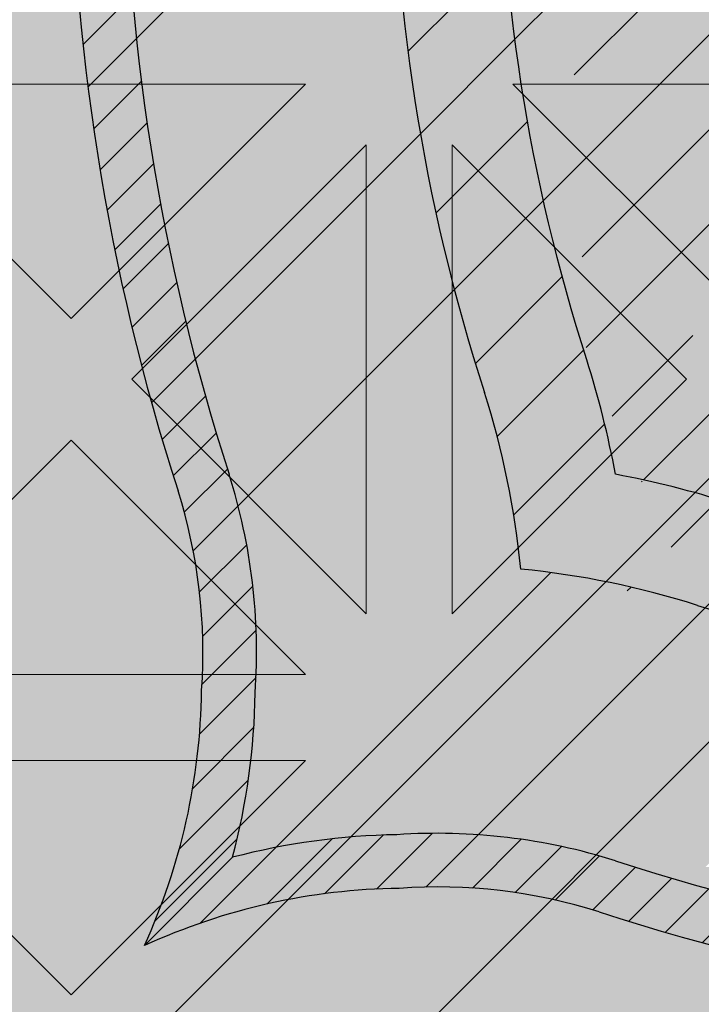
# Model space of a CAD drawing. Units: inches. Extents: x 844 to 2234, y 346 to 1084.
# Tile 10 of 93: x 1119.118 to 1121.143, y 688.258 to 691.183. Entities that reach past the tile are written whole.
import ezdxf

# ---------------------------------------------------------------- set-up
doc = ezdxf.new("R2010")
doc.units = ezdxf.units.IN
doc.header["$MEASUREMENT"] = 0
for name, color, linetype, lineweight in [('A-ANNO-DIMS', 2, 'Continuous', 18), ('furniture', 8, 'Continuous', 18), ('RA-AP-01$0$INT', 35, 'Continuous', 5)]:
    doc.layers.add(name, color=color, linetype=linetype, lineweight=lineweight)
doc.layers.add('RA-AP-01$0$FURN', color=3, linetype='Continuous')
doc.layers.add('RA-AP-01$0$WOOD', color=64, linetype='Continuous')
doc.styles.get("Standard").update_dxf_attribs({"font": 'arial.ttf'})
doc.dimstyles.get("Standard").update_dxf_attribs({"dimtxt": 6, "dimasz": 3, "dimexe": 0.18, "dimexo": 0.0625, "dimgap": 0.09, "dimtad": 0, "dimtih": 1, "dimtoh": 1, "dimdec": 1, "dimzin": 0, "dimdsep": 46, "dimlunit": 3, "dimtxsty": 'Standard', "dimblk": 'ARCHTICK', "dimcen": 0.09, "dimadec": 0, "dimazin": 0, "dimtfac": 1, "dimtdec": 1, "dimtofl": 0, "dimtmove": 0, "dimatfit": 3, "dimfxl": 1, "dimtolj": 1, "dimtzin": 0, "dimarcsym": 0})

# ---------------------------------------------------------------- blocks, each defined once
blk = doc.blocks.new('A$C18D01794')
at = {"layer": 'RA-AP-01$0$INT'}
h = blk.add_hatch(color=256, dxfattribs=at)
h.paths.add_polyline_path([(4.585917135068449, -6.356712009588271), (4.555206456959269, -6.35671200958746), (4.555206456959137, -6.387422687716308), (4.874495778835233, -6.706712009592356), (4.90520645695423, -6.676001331474049)])
h.paths.add_polyline_path([(5.255206456948813, -6.387422687716306), (5.255206456948682, -6.356712009605972), (5.224495778822613, -6.356712009605161), (4.905206456953498, -6.676001331474273), (4.935917135072151, -6.706712009592924)])
h.paths.add_polyline_path([(4.935917135072559, -6.706712009592068), (4.905206456953564, -6.737422687710376), (5.255206456951813, -7.087422687708613), (5.255206456951549, -7.026001331471008)])
h.paths.add_polyline_path([(4.555206456956399, -7.026001331471013), (4.555206456956134, -7.087422687708616), (4.905206456953821, -6.737422687710943), (4.874495778835166, -6.70671200959229)])
h = blk.add_hatch(color=256, dxfattribs=at)
h.paths.add_polyline_path([(4.585917135068448, -6.356712009588273), (4.614201406330596, -6.356712009589021), (4.668846067270487, -6.411356670531338), (4.723490728212344, -6.356712009591912), (4.771774999457151, -6.35671200959319), (4.826419660396886, -6.411356670535356), (4.862780050090322, -6.374996280843536), (4.844495778842715, -6.356712009595112), (4.862780050090411, -6.356712009595595), (4.905206456960182, -6.399138416468211), (4.947632863832445, -6.356712009597838), (4.965917135079675, -6.356712009598322), (4.947632863831759, -6.374996280845421), (4.983993253523576, -6.411356670538857), (5.038637914464627, -6.356712009600247), (5.08692218571208, -6.356712009601523), (5.141566846649976, -6.411356670541852), (5.196211507589851, -6.356712009604411), (5.224495778822615, -6.356712009605161), (4.905206456953975, -6.676001331473793)])
h.paths.add_polyline_path([(4.895206456956031, -6.637717060225675), (4.895206456958921, -6.528427738347902), (4.840561796018589, -6.583072399285802)], flags=16)
h.paths.add_polyline_path([(4.915206456955638, -6.637717060226121), (4.969851117895509, -6.583072399288678), (4.915206456957609, -6.528427738348344)], flags=16)
h.paths.add_polyline_path([(4.826419660395175, -6.568930263661755), (4.881064321335613, -6.514285602723745), (4.771774999456703, -6.514285602720857)], flags=16)
h.paths.add_polyline_path([(4.983993253519558, -6.568930263665262), (5.038637914460456, -6.514285602726792), (4.929348592581548, -6.514285602724816)], flags=16)
h.paths.add_polyline_path([(4.881064321336025, -6.494285602723742), (4.826419660397532, -6.439640941782821), (4.771774999457062, -6.494285602720859)], flags=16)
h.paths.add_polyline_path([(4.929348592582019, -6.494285602724817), (5.038637914460982, -6.494285602726792), (4.983993253522945, -6.439640941786327)], flags=16)
h.paths.add_polyline_path([(4.895206456960191, -6.480143467100443), (4.895206456962115, -6.407422687715913), (4.876922185715016, -6.389138416467584), (4.840561796021581, -6.425498806159401)], flags=16)
h.paths.add_polyline_path([(4.915206456958487, -6.480143467100889), (4.969851117899527, -6.425498806162279), (4.933490728206909, -6.389138416468043), (4.9152064569598, -6.40742268771434)], flags=16)
h.paths.add_polyline_path([(4.757632863832376, -6.480143467096812), (4.812277524772842, -6.425498806158772), (4.757632863834348, -6.370854145217844)], flags=16)
h.paths.add_polyline_path([(4.737632863832376, -6.480143467096286), (4.737632863834348, -6.370854145217375), (4.682988202893906, -6.425498806155385)], flags=16)
h.paths.add_polyline_path([(5.05278005008503, -6.480143467103376), (5.052780050087917, -6.370854145224413), (4.998135389146995, -6.425498806162908)], flags=16)
h.paths.add_polyline_path([(5.072780050085024, -6.480143467103744), (5.127424711025931, -6.42549880616527), (5.072780050087916, -6.370854145224832)], flags=16)
h.paths.add_polyline_path([(4.935917135072783, -6.706712009592292), (5.255206456948811, -6.387422687716309), (5.255206456948932, -6.415706958964177), (5.200561796010279, -6.470351619902839), (5.255206456949403, -6.524996280841948), (5.25520645694961, -6.5732805520894), (5.200561796009787, -6.627925213029239), (5.236922185702417, -6.664285602721864), (5.255206456949919, -6.646001331474357), (5.255206456949998, -6.664285602721898), (5.212780050078687, -6.706712009592262), (5.25520645695036, -6.749138416463932), (5.255206456950438, -6.767422687711313), (5.236922185702424, -6.749138416463297), (5.200561796009796, -6.785498806155928), (5.255206456950753, -6.840143467096874), (5.25520645695096, -6.888427738341682), (5.200561796010322, -6.943072399282328), (5.255206456951428, -6.997717060223427), (5.255206456951547, -7.026001331471006)])
h.paths.add_polyline_path([(5.042988202883395, -6.785498806155427), (5.097632863823085, -6.840143467095101), (5.097632863822622, -6.730854145216193)], flags=16)
h.paths.add_polyline_path([(5.028846067259663, -6.771356670531693), (5.083490728198774, -6.716712009592573), (4.974201406321001, -6.716712009593042)], flags=16)
h.paths.add_polyline_path([(5.117632863823087, -6.840143467095186), (5.172277524762331, -6.785498806155926), (5.11763286382262, -6.730854145216225)], flags=16)
h.paths.add_polyline_path([(5.08349072819877, -6.696712009593886), (5.028846067259652, -6.642067348654775), (4.974201406320998, -6.696712009593438)], flags=16)
h.paths.add_polyline_path([(5.131774999446817, -6.854285602718917), (5.186419660386065, -6.799640941779662), (5.241064321325782, -6.854285602719365)], flags=17)
h.paths.add_polyline_path([(5.131774999446228, -6.716712009592374), (5.186419660386065, -6.771356670532194), (5.222780050079488, -6.734996280838764), (5.204495778832781, -6.716712009592063)], flags=16)
h.paths.add_polyline_path([(5.097632863822613, -6.682569873970264), (5.097632863823061, -6.573280552091354), (5.042988202883383, -6.627925213031044)], flags=16)
h.paths.add_polyline_path([(5.131774999446899, -6.874285602718915), (5.241064321325809, -6.874285602719364), (5.186419660386591, -6.928930263658598)], flags=17)
h.paths.add_polyline_path([(5.131774999446226, -6.696712009594078), (5.204495778830767, -6.696712009594374), (5.22278005007868, -6.67842773834687), (5.186419660386049, -6.642067348654249)], flags=16)
h.paths.add_polyline_path([(5.11763286382262, -6.682569873970225), (5.17227752476232, -6.627925213030515), (5.117632863823064, -6.573280552091267)], flags=16)
h.paths.add_polyline_path([(5.186419660386069, -6.613783077405491), (5.241064321325754, -6.559138416465795), (5.131774999446791, -6.559138416466263)], flags=16)
h.paths.add_polyline_path([(5.131774999446872, -6.539138416466263), (5.24106432132578, -6.539138416465794), (5.186419660386554, -6.484493755526573)], flags=16)
h.paths.add_polyline_path([(5.255206456951811, -7.08742268770861), (5.255206456951895, -7.106712009588038), (4.555206456956052, -7.106712009588038), (4.555206456956136, -7.087422687708617), (4.905206456953973, -6.737422687710788)])
h.paths.add_polyline_path([(4.983993253513404, -6.8444937555241), (4.92934859257295, -6.899138416462108), (5.03863791445186, -6.899138416465014)], flags=16)
h.paths.add_polyline_path([(4.969851117889988, -6.83035161990006), (4.915206456952556, -6.775706958960171), (4.915206456949648, -6.884996280837944)], flags=16)
h.paths.add_polyline_path([(4.929348592572535, -6.919138416462105), (4.983993253511019, -6.973783077403037), (5.038637914451496, -6.919138416465012)], flags=16)
h.paths.add_polyline_path([(5.052780050074912, -6.93328055208906), (4.998135389134438, -6.987925213027088), (5.052780050072919, -7.042569873968025)], flags=16)
h.paths.add_polyline_path([(5.07278005007491, -6.933280552089588), (5.072780050072918, -7.042569873968497), (5.127424711013374, -6.987925213030498)], flags=16)
h.paths.add_polyline_path([(4.89520645695295, -6.775706958959721), (4.840561796013067, -6.830351619897157), (4.895206456950961, -6.884996280837494)], flags=16)
h.paths.add_polyline_path([(4.915206456948365, -6.933280552085403), (4.915206456946434, -7.006001331471951), (4.933490728192729, -7.024285602719066), (4.969851117886972, -6.987925213026453)], flags=16)
h.paths.add_polyline_path([(4.881064321327021, -6.899138416461022), (4.82641966038902, -6.84449375552057), (4.771774999448108, -6.899138416459029)], flags=16)
h.paths.add_polyline_path([(4.895206456950073, -6.933280552084951), (4.840561796009022, -6.987925213023558), (4.876922185700835, -7.024285602716997), (4.895206456948749, -7.006001331469487)], flags=16)
h.paths.add_polyline_path([(4.983993253510392, -7.0020673486505), (4.947632863816944, -7.038427738342319), (4.965917135064043, -7.05671200959023), (5.038637914448995, -7.056712009591555)], flags=16)
h.paths.add_polyline_path([(4.881064321326543, -6.91913841646102), (4.771774999447578, -6.919138416459031), (4.826419660385607, -6.973783077399508)], flags=16)
h.paths.add_polyline_path([(4.905206456946447, -7.014285602717636), (4.862780050074785, -7.056712009588352), (4.947632863816685, -7.056712009589775)], flags=16)
h.paths.add_polyline_path([(5.14156684663679, -7.002067348654549), (5.086922185696452, -7.056712009592438), (5.196211507574223, -7.056712009594425)], flags=16)
h.paths.add_polyline_path([(4.8264196603837, -7.002067348646972), (4.771774999442643, -7.056712009585575), (4.8444957788276, -7.056712009587508), (4.862780050075511, -7.038427738340416)], flags=16)
h.paths.add_polyline_path([(4.812277524760289, -6.98792521302292), (4.757632863822258, -6.933280552082447), (4.757632863819352, -7.042569873961408)], flags=16)
h.paths.add_polyline_path([(4.73763286382226, -6.933280552082079), (4.682988202881349, -6.987925213020536), (4.737632863819352, -7.04256987396099)], flags=16)
h.paths.add_polyline_path([(4.723490728195188, -7.056712009584289), (4.668846067257299, -7.002067348643949), (4.614201406317417, -7.056712009581383)], flags=16)
h.paths.add_polyline_path([(4.597632863829262, -6.706712009592262), (4.555206456957951, -6.664285602721896), (4.555206456958029, -6.646001331474357), (4.573490728205535, -6.664285602721864), (4.609851117898167, -6.627925213029238), (4.555206456958338, -6.573280552089402), (4.555206456958546, -6.524996280841952), (4.60985111789767, -6.470351619902839), (4.555206456959015, -6.415706958964177), (4.555206456959138, -6.387422687716309), (4.874495778835167, -6.70671200959229), (4.5552064569564, -7.026001331471015), (4.555206456956523, -6.997717060223433), (4.609851117897629, -6.94307239928233), (4.555206456956988, -6.888427738341681), (4.555206456957198, -6.840143467096881), (4.609851117898153, -6.78549880615593), (4.573490728205528, -6.749138416463297), (4.555206456957507, -6.76742268771132), (4.555206456957585, -6.749138416463933)])
h.paths.add_polyline_path([(4.712780050085332, -6.730854145216195), (4.712780050084863, -6.840143467095105), (4.767424711024555, -6.785498806155427)], flags=16)
h.paths.add_polyline_path([(4.726922185709173, -6.716712009592573), (4.781566846648288, -6.771356670531693), (4.836211507586949, -6.716712009593043)], flags=16)
h.paths.add_polyline_path([(4.692780050085327, -6.730854145216225), (4.638135389145619, -6.785498806155928), (4.692780050084865, -6.840143467095185)], flags=16)
h.paths.add_polyline_path([(4.726922185709182, -6.696712009593886), (4.836211507586949, -6.696712009593436), (4.7815668466483, -6.642067348654773)], flags=16)
h.paths.add_polyline_path([(4.678637914461726, -6.71671200959237), (4.605917135075169, -6.716712009592063), (4.587632863828464, -6.734996280838766), (4.623993253521887, -6.771356670532195)], flags=16)
h.paths.add_polyline_path([(4.712780050085336, -6.68256987397026), (4.767424711024568, -6.627925213031042), (4.71278005008489, -6.573280552091352)], flags=16)
h.paths.add_polyline_path([(4.678637914461726, -6.696712009594076), (4.623993253521899, -6.642067348654247), (4.587632863829271, -6.67842773834687), (4.605917135077185, -6.696712009594376)], flags=16)
h.paths.add_polyline_path([(4.692780050085336, -6.682569873970228), (4.692780050084889, -6.573280552091267), (4.638135389145632, -6.627925213030515)], flags=16)
h.paths.add_polyline_path([(4.623993253521885, -6.799640941779662), (4.678637914461131, -6.854285602718915), (4.56934859258217, -6.854285602719365)], flags=17)
h.paths.add_polyline_path([(4.623993253521901, -6.613783077405509), (4.678637914461158, -6.559138416466263), (4.569348592582195, -6.559138416465795)], flags=16)
h.paths.add_polyline_path([(4.678637914461051, -6.874285602718915), (4.623993253521361, -6.928930263658598), (4.569348592582143, -6.874285602719364)], flags=17)
h.paths.add_polyline_path([(4.678637914461076, -6.539138416466263), (4.623993253521399, -6.484493755526573), (4.569348592582167, -6.539138416465796)], flags=16)
h = blk.add_hatch(color=256, dxfattribs=at)
h.paths.add_polyline_path([(4.781566846647504, -6.771356670530272), (4.836211507586161, -6.716712009591613), (4.726922185708388, -6.716712009591159)])
h.paths.add_polyline_path([(4.836211507586161, -6.696712009592008), (4.781566846647504, -6.642067348653354), (4.726922185708388, -6.69671200959247)])
h.paths.add_polyline_path([(4.76742471102377, -6.627925213029623), (4.712780050084083, -6.57328055208994), (4.712780050084542, -6.68256987396885)])
h.paths.add_polyline_path([(4.692780050084544, -6.682569873968819), (4.692780050084084, -6.573280552089856), (4.638135389144834, -6.627925213029111)])
h.paths.add_polyline_path([(4.678637914460932, -6.696712009592669), (4.623993253521102, -6.642067348652844), (4.587632863827676, -6.678427738346266), (4.605917135074382, -6.696712009592973)])
h.paths.add_polyline_path([(4.573490728204743, -6.664285602721736), (4.60985111789737, -6.627925213029108), (4.555206456957541, -6.573280552089279), (4.555206456957237, -6.646001331474231)])
h.paths.add_polyline_path([(4.623993253521098, -6.613783077405377), (4.67863791446035, -6.559138416466126), (4.56934859258139, -6.559138416465669)])
h.paths.add_polyline_path([(4.678637914460275, -6.539138416466126), (4.623993253520583, -6.48449375552644), (4.56934859258136, -6.539138416465672)])
h.paths.add_polyline_path([(4.609851117896854, -6.470351619902707), (4.555206456958196, -6.415706958964051), (4.555206456957738, -6.524996280841822)])
h.paths.add_polyline_path([(4.597632863828475, -6.706712009592775), (4.555206456957283, -6.664285602721582), (4.555206456956805, -6.749138416463489)])
h.paths.add_polyline_path([(4.678637914460932, -6.716712009590963), (4.605917135076396, -6.71671200959066), (4.587632863828479, -6.734996280838164), (4.623993253521104, -6.771356670530792)])
h.paths.add_polyline_path([(4.692780050084091, -6.840143467093776), (4.692780050084548, -6.730854145214809), (4.638135389144834, -6.785498806154524)])
h.paths.add_polyline_path([(4.767424711023772, -6.785498806154004), (4.712780050084545, -6.730854145214786), (4.712780050084089, -6.840143467093692)])
h.paths.add_polyline_path([(4.67863791446036, -6.854285602718778), (4.623993253521105, -6.799640941779527), (4.569348592581399, -6.854285602719237)])
h.paths.add_polyline_path([(4.609851117897371, -6.785498806155798), (4.573490728204743, -6.74913841646317), (4.555206456957237, -6.767422687710675), (4.555206456957548, -6.840143467095629)])
h.paths.add_polyline_path([(4.623993253520596, -6.928930263658465), (4.67863791446028, -6.874285602718778), (4.569348592581367, -6.874285602719238)])
h.paths.add_polyline_path([(4.609851117896867, -6.943072399282199), (4.555206456957749, -6.888427738343082), (4.55520645695821, -6.997717060220857)])
for p, q in [((4.905206456953975, -6.676001331473793), (4.585917135071132, -6.356712009590955)), ((4.874495778835167, -6.70671200959229), (4.555206456959136, -6.387422687716307)), ((4.569348592582168, -6.539138416465796), (4.623993253521399, -6.484493755526573)), ((4.6239932535214, -6.484493755526575), (4.678637914461078, -6.539138416466263)), ((4.678637914461078, -6.539138416466263), (4.569348592582168, -6.539138416465796)), ((4.569348592582195, -6.559138416465795), (4.623993253521901, -6.613783077405509)), ((4.678637914461158, -6.559138416466263), (4.569348592582195, -6.559138416465795)), ((4.678637914461158, -6.559138416466263), (4.623993253521901, -6.613783077405509)), ((4.692780050084889, -6.573280552091267), (4.638135389145632, -6.627925213030515)), ((4.692780050084889, -6.573280552091267), (4.692780050085336, -6.68256987397023)), ((4.767424711024566, -6.627925213031041), (4.712780050084888, -6.573280552091352)), ((4.712780050084888, -6.573280552091352), (4.712780050085336, -6.682569873970262)), ((4.692780050085336, -6.68256987397023), (4.638135389145632, -6.627925213030515)), ((4.712780050085336, -6.682569873970262), (4.767424711024568, -6.627925213031042)), ((4.623993253521899, -6.642067348654247), (4.587632863829269, -6.67842773834687)), ((4.678637914461723, -6.696712009594078), (4.623993253521898, -6.642067348654247)), ((4.726922185709182, -6.696712009593882), (4.781566846648298, -6.642067348654775)), ((4.605917135076771, -6.696712009594376), (4.678637914461723, -6.696712009594078)), ((4.72692218570918, -6.696712009593886), (4.836211507586951, -6.696712009593436))]:
    blk.add_line(p, q, dxfattribs=at)
blk = doc.blocks.new('A$C32926AE1')
at = {"layer": 'RA-AP-01$0$FURN'}
h = blk.add_hatch(dxfattribs=at)
h.set_pattern_fill('ANSI31', color=256, scale=0.1, style=0)
h.set_pattern_definition([(45, (0, 0), (-0.0088388347648318, 0.0088388347648318), [])])
edge = h.paths.add_edge_path(flags=16)
edge.add_arc((4.904771284329206, 4.246793130718756), 0.2603971832811541, 75.22398030683196, 104.7760196931204)
edge.add_arc((4.904771284329206, 4.246793130718756), 0.2603971832811541, 75.223980306832, 104.77601969312039, ccw=False)
edge = h.paths.add_edge_path(flags=16)
edge.add_arc((4.904771284329206, 4.067062675376612), 0.2603971832811541, 255.2239803068796, 284.776019693168)
edge.add_arc((4.904771284329206, 4.067062675376612), 0.2603971832811541, 255.22398030687958, 284.77601969316805, ccw=False)
edge = h.paths.add_edge_path(flags=0)
edge.add_arc((4.904771284329206, 4.067062675376612), 0.2603971832811541, 255.2239803068796, 284.776019693168)
edge.add_arc((4.904771284329206, 4.067062675376612), 0.2603971832811541, 255.22398030687958, 284.77601969316805, ccw=False)
edge = h.paths.add_edge_path(flags=0)
edge.add_arc((4.904771284329206, 4.067062675376612), 0.2603971832811541, 255.2239803068796, 284.776019693168)
edge.add_arc((4.904771284329206, 4.067062675376612), 0.2603971832811541, 255.22398030687958, 284.77601969316805, ccw=False)
edge = h.paths.add_edge_path()
edge.add_arc((4.604388392048174, 4.588829985554312), 0.1599999999999918, 342.3781640246255, 354.4317409793762)
edge.add_arc((5.090145208887507, 4.43216705527679), 0.3503971832811637, 162.0091218307731, 180.3186872093483)
edge.add_arc((5.205154176610243, 4.588829985554953), 0.1599999999999917, 185.5682590208461, 197.6218359767349)
edge.add_arc((4.904771284329229, 4.246793130718735), 0.3503971832811761, 72.00912183053516, 107.9908781690354)
edge.add_arc((9.535952835716557, 4.28682295566602), 4.798342501046485, 178.2875002453811, 181.5576802719453)
edge.add_arc((4.719397359771122, 4.43216705527679), 0.3503971832811637, 359.6813127906516, 377.9908781692269)
edge.add_arc((9.535967292294904, 4.286822350292874), 4.778371420254705, 178.2965938931842, 181.5667745797229)
edge.add_arc((4.719397359771122, 4.43216705527679), 0.3303971832811637, 359.6813127906516, 377.9908781692269)
edge.add_arc((0.2735752763637294, 4.286822350292874), 4.7783714202547, 358.4332254202771, 361.7034061068158)
edge.add_arc((5.061434214606998, 4.732549947558029), 0.1600000000000254, 252.3781640250584, 264.4317409792362)
edge.add_arc((4.748108354051257, 4.732549947558012), 0.1600000000000541, 275.5682590208426, 287.6218359759532)
edge.add_arc((4.604388392048115, 4.588829985554317), 0.1800000000000505, 342.3567572500182, 349.3735009646207)
edge.add_arc((5.205154176610254, 4.588829985554976), 0.1800000000000069, 190.6264990356027, 197.6432427513933)
edge.add_arc((5.061434214607106, 4.732549947558013), 0.1800000000000424, 252.3567572496606, 259.3735009644582)
edge.add_arc((4.904771284329208, 4.246793130718737), 0.3303971832811676, 71.99844483668534, 108.0015551637021)
edge.add_arc((4.748108354051414, 4.732549947558045), 0.1800000000000547, 280.6264990355479, 287.6432427495938)
edge.add_arc((5.090145208887514, 4.432167055276789), 0.2803971832811691, 162.8706300666893, 180.816523289902)
edge.add_arc((4.719397359771136, 4.432167055276689), 0.2803971832811534, 359.183476710103, 377.1293699333214)
edge.add_arc((4.904771284329222, 4.246793130718737), 0.2803971832811769, 72.87063006672916, 107.1293699332334)
edge.add_arc((5.090145208887522, 4.432167055276788), 0.2603971832811776, 165.2239803068007, 180.9953123810312)
edge.add_arc((4.719397359771141, 4.432167055276699), 0.2603971832811458, 359.0046876189768, 374.7760196932087)
edge.add_arc((5.090145208887507, 4.43216705527679), 0.3303971832811637, 162.0091218307731, 180.3186872093483)
edge.add_arc((9.53595427642584, 4.285015535491528), 4.728345371032053, 178.265043920078, 181.5679956281801)
edge.add_arc((0.2735882922327999, 4.285015535491582), 4.728345371032045, 358.4320043718193, 361.7349560799204)
edge.add_arc((9.535953591267507, 4.284458026472751), 4.708343996644348, 178.2573054306777, 181.5704995759608)
edge.add_arc((0.273588977391114, 4.284458026472785), 4.708343996644358, 358.4295004240388, 361.7426945693213)
edge.add_arc((0.2735889773911131, 4.029397779622582), 4.708343996644359, 358.2573054306787, 361.5704995759613)
edge.add_arc((9.535953591267518, 4.029397779622618), 4.708343996644359, 178.4295004240391, 181.7426945693223)
edge.add_arc((0.2735882922327901, 4.028840270603786), 4.728345371032054, 358.2650439200796, 361.5679956281808)
edge.add_arc((9.53595427642584, 4.028840270603841), 4.728345371032054, 178.4320043718199, 181.7349560799219)
edge.add_arc((0.2735752763637302, 4.027033455802493), 4.778371420254699, 358.2965938931842, 361.5667745797229)
edge.add_arc((4.719397359771122, 3.881688750818578), 0.3303971832811637, 342.0091218307731, 360.3186872093484)
edge.add_arc((5.090145208887507, 3.881688750818578), 0.3303971832811637, 179.6813127906516, 197.9908781692269)
edge.add_arc((9.535967292294904, 4.027033455802493), 4.778371420254705, 178.433225420277, 181.7034061068158)
edge.add_arc((4.719397359771122, 3.881688750818578), 0.3503971832811637, 342.0091218307731, 360.3186872093484)
edge.add_arc((9.53595283571655, 4.027032850429349), 4.79834250104648, 178.4423197280546, 181.7124997546188)
edge.add_arc((4.719397359771141, 3.881688750818669), 0.2603971832811458, 345.2239803067913, 360.9953123810232)
edge.add_arc((5.090145208887522, 3.88168875081858), 0.2603971832811776, 179.0046876189687, 194.7760196931993)
edge.add_arc((4.904771284329222, 4.067062675376631), 0.2803971832811769, 252.8706300667665, 287.1293699332708)
edge.add_arc((4.719397359771136, 3.881688750818678), 0.2803971832811534, 342.8706300666787, 360.8165232898969)
edge.add_arc((5.090145208887514, 3.881688750818579), 0.2803971832811691, 179.183476710098, 197.1293699333106)
edge.add_arc((4.748108354051414, 3.581305858537323), 0.1800000000000547, 72.3567572504062, 79.37350096445199)
edge.add_arc((4.904771284329208, 4.067062675376631), 0.3303971832811676, 251.9984448362979, 288.0015551633146)
edge.add_arc((5.061434214607106, 3.581305858537355), 0.1800000000000424, 100.6264990355418, 107.6432427503394)
edge.add_arc((5.205154176610254, 3.725025820540392), 0.1800000000000069, 162.3567572486066, 169.3735009643972)
edge.add_arc((4.604388392048115, 3.725025820541051), 0.1800000000000505, 10.62649903537925, 17.64324274998182)
edge.add_arc((4.748108354051257, 3.581305858537356), 0.1600000000000541, 72.37816402404681, 84.43174097915735)
edge.add_arc((4.904771284329229, 4.067062675376632), 0.3503971832811761, 252.0091218309645, 287.9908781694648)
edge.add_arc((5.061434214606998, 3.581305858537339), 0.1600000000000254, 95.56825902076373, 107.6218359749416)
edge.add_arc((5.205154176610243, 3.725025820540414), 0.1599999999999917, 162.3781640232651, 174.4317409791539)
edge.add_arc((5.090145208887507, 3.881688750818578), 0.3503971832811637, 179.6813127906516, 197.9908781692269)
edge.add_arc((4.604388392048174, 3.725025820541056), 0.1599999999999918, 5.568259020623824, 17.62183597537444)
edge.add_arc((0.2735897329420762, 4.28682295566602), 4.798342501046482, 358.4423197280547, 361.7124997546188)
edge.add_arc((0.2735897329420691, 4.027032850429348), 4.798342501046489, 358.2875002453812, 361.5576802719453)
at = {"layer": 'RA-AP-01$0$WOOD'}
h = blk.add_hatch(color=256, dxfattribs=at)
h.dxf.hatch_style = 1
h.paths.add_polyline_path([(5.157430609644524, 4.573483066760929, -0.1009492694046607), (5.155401577623758, 4.593365984175333, -0.1842662638101597), (5.172249623284174, 4.638795604568598, 0.2056608120311276), (5.179560981299304, 4.661316324430096, 0.3614336704623542), (5.134352340494423, 4.706524965234944, 0.2056608120311297), (5.111831620632933, 4.699213607219793, -0.1842662638101113), (5.066402000239693, 4.682365561559342, -0.1055311479399994), (5.045656153913092, 4.68467289944697, 0.1567636581983829), (4.763886414745334, 4.684672899446966, -0.1055311479399895), (4.743140568418733, 4.68236556155934, -0.1842662638100833), (4.6977109480255, 4.69921360721979, 0.2056608120302612), (4.675190228164109, 4.706524965234949, 0.3614336704708441), (4.629981587358889, 4.66131632442871, 0.2056608120245944), (4.637292945374126, 4.638795604567974, -0.1842662638101024), (4.654140991034615, 4.59336598417475, -0.1009492694055169), (4.652111959013835, 4.573483066760181, 0.021410119221476), (4.629748025606143, 4.156712009541676, 0.0214101192214795), (4.652111959013809, 3.739940952323101, -0.1009492694059586), (4.654140991034615, 3.720058034908448, -0.1842662638100975), (4.637292945374126, 3.674628414515226, 0.2056608120245705), (4.629981587358889, 3.652107694654492, 0.3614336704708879), (4.675190228164113, 3.606899053848249, 0.2056608120302384), (4.697710948025501, 3.614210411863408, -0.1842662638100995), (4.743140568418738, 3.63105845752386, -0.1055311479402541), (4.763886414745388, 3.628751119636215, 0.1567636581983776), (5.045656153913137, 3.628751119636244, -0.1055311479397538), (5.066402000239692, 3.631058457523857, -0.1842662638101067), (5.111831620632931, 3.614210411863407, 0.2056608120310924), (5.134352340494417, 3.606899053848256, 0.3614336704624001), (5.179560981299307, 3.652107694653103, 0.2056608120311314), (5.172249623284175, 3.6746284145146, -0.1842662638101402), (5.155401577623758, 3.72005803490786, -0.1009492694051366), (5.15743060964455, 3.739940952322354, 0.0214101192215073), (5.179794543052287, 4.156712009541468, 0.0214101192215252)])
h.paths.add_polyline_path([(4.639748609479751, 4.156712009541513, 0.0213537860821624), (4.661970494867118, 3.741887061152232, -0.094075836301374), (4.664143710413708, 3.7196126951003, -0.1824818158568985), (4.644813765429836, 3.668037719127816, 0.2056608120245319), (4.639939526753007, 3.653023905887301, 0.3614336704710246), (4.676106439397173, 3.616856993242342, 0.2056608120302234), (4.691120252638095, 3.621731231919122, -0.1824818158602558), (4.742695228611606, 3.641061176902986, -0.1029891339458722), (4.766991894714349, 3.638256818950944, 0.156709409989566), (5.042550673941472, 3.638256818950105, -0.102989133958497), (5.066847340047078, 3.641061176902949, -0.1824818158594995), (5.118422316020358, 3.621731231919103, 0.2056608120311416), (5.133436129261316, 3.616856993242346, 0.3614336704621468), (5.169603041905217, 3.653023905886178, 0.2056608120310986), (5.164728803228477, 3.668037719127177, -0.1824818158565612), (5.145398858244737, 3.719612695099578, -0.0940758363009313), (5.147572073791232, 3.741887061151398, 0.0213537860822023), (5.169793959178681, 4.156712009541451, 0.0213537860822226), (5.147572073791203, 4.571536957931898, -0.0940758363005034), (5.145398858244737, 4.59381132398362, -0.1824818158565587), (5.164728803228476, 4.645386299956021, 0.2056608120311045), (5.169603041905216, 4.66040011319702, 0.3614336704621845), (5.133436129261313, 4.696567025840856, 0.2056608120310773), (5.118422316020359, 4.691692787164098, -0.182481815859508), (5.066847340047078, 4.67236284218025, -0.1029891339584606), (5.04255067394148, 4.675167200133092, 0.156709409989566), (4.766991894714357, 4.675167200132257, -0.1029891339458842), (4.742695228611611, 4.672362842180213, -0.1824818158602725), (4.691120252638095, 4.691692787164077, 0.2056608120302152), (4.676106439397174, 4.696567025840858, 0.3614336704710363), (4.639939526753005, 4.660400113195899, 0.2056608120245495), (4.644813765429837, 4.645386299955384, -0.1824818158568934), (4.664143710413708, 4.593811323982902, -0.0940758363009187), (4.661970494867149, 4.571536957931074, 0.021353786082177)], flags=16)
h.paths.add_polyline_path([(5.129794543052235, 4.432167055276933, -0.0141661062790638), (5.130152669293814, 4.156927903047693, -0.0141661062790647), (5.129794543052234, 3.881688750818433, -0.0785247771143638), (5.10979738006795, 3.755143611847103, 0.0945969212073497), (5.105408519571111, 3.717898134952927, 0.1043170707844957), (5.116074640131521, 3.670385395016088, 0.1043170707864965), (5.068561900193738, 3.681051515576561, 0.09459692119553), (5.031316423304057, 3.676662655080835, -0.1580239521427272), (4.778226145355827, 3.676662655080367, 0.0945969211986668), (4.740980668464973, 3.681051515576592, 0.1043170707882822), (4.693467928526415, 3.670385395015844, 0.1043170707867916), (4.704134049087309, 3.717898134953662, 0.0945969211972894), (4.69974518859162, 3.755143611844042, -0.0785247771163196), (4.679748025606343, 3.881688750818406, -0.0141661062790663), (4.679389899364763, 4.156927903047693, -0.0141661062790672), (4.679748025606343, 4.432167055276998, -0.0785247771163064), (4.699745188591625, 4.55871219425134, 0.094596921197333), (4.704134049087308, 4.595957671141738, 0.1043170707867205), (4.693467928526416, 4.643470411079523, 0.1043170707882628), (4.740980668464965, 4.632804290518776, 0.0945969211988114), (4.778226145355874, 4.637193151015016, -0.158023952142669), (5.031316423304015, 4.637193151014546, 0.0945969211956361), (5.068561900193736, 4.632804290518806, 0.1043170707864979), (5.11607464013152, 4.643470411079278, 0.1043170707844617), (5.105408519571112, 4.595957671142455, 0.0945969212074597), (5.109797380067959, 4.558712194248236, -0.0785247771143467)], flags=0)
h.paths.add_polyline_path([(5.119794532311105, 4.432259799204851, -0.0142000800617244), (5.120156169157484, 4.156927903047701, -0.0142000800617277), (5.119794532311105, 3.881596006890482, -0.0784894509520253), (5.100273383573699, 3.758192358677797, 0.0940138827242913), (5.095413455884425, 3.717477693979438, 0.0606271852308753), (5.099615656341024, 3.686844378806616, 0.0606271852322524), (5.068982341167493, 3.691046579263239, 0.0940138827010453), (5.028267676478798, 3.686186651576848, -0.1580706864508061), (4.781274892180912, 3.686186651576435, 0.0940138827026903), (4.740560227491556, 3.691046579263279, 0.0606271852339895), (4.709926912317155, 3.686844378806508, 0.0606271852329405), (4.714129112773991, 3.717477693980356, 0.094013882701304), (4.709269185087677, 3.758192358669163, -0.0784894509577193), (4.689748036347473, 3.881596006890469, -0.014200080061729), (4.689386399501094, 4.156927903047709, -0.0142000800617217), (4.689748036347473, 4.432259799204808, -0.078489450957724), (4.709269185087651, 4.555663447426125, 0.0940138827014585), (4.714129112773992, 4.596378112114996, 0.0606271852329731), (4.709926912317154, 4.62701142728886, 0.0606271852340196), (4.74056022749157, 4.622809226832087, 0.0940138827024997), (4.781274892180847, 4.627669154518912, -0.1580706864508359), (5.028267676478777, 4.627669154518526, 0.0940138827010946), (5.068982341167492, 4.622809226832129, 0.060627185232254), (5.099615656341024, 4.627011427288751, 0.0606271852308727), (5.095413455884425, 4.59637811211593, 0.0940138827241088), (5.100273383573675, 4.555663447417647, -0.0784894509520978)], flags=0)
h.paths.add_polyline_path([(5.06978912287499, 4.430218106756144, -0.014241683694547), (5.070173729147532, 4.156927903047672, -0.0142416836945458), (5.06978912287499, 3.883637699339223, -0.0800609523125196), (5.052662118612511, 3.773463122773442, 0.0526421978001116), (5.04590916754064, 3.740550867606997, 0.0526421977992423), (5.012996912374707, 3.73379791653534, -0.1583028414718258), (4.796545656286308, 3.73379791653451, 0.0526421978034211), (4.763633401117837, 3.740550867607021, 0.0526421978018622), (4.756880450045755, 3.773463122774558, -0.0800609523117106), (4.739753445783639, 3.883637699339268, -0.0142416836945435), (4.739368839511098, 4.156927903047671, -0.0142416836945477), (4.739753445783639, 4.430218106756155, -0.0800609523116345), (4.75688045004574, 4.540392683320762, 0.052642197801941), (4.763633401117837, 4.573304938488346, 0.0526421978035071), (4.796545656286361, 4.580057889560873, -0.1583028414717561), (5.012996912374669, 4.580057889560039, 0.0526421977993048), (5.04590916754064, 4.57330493848837, 0.0526421978002057), (5.052662118612529, 4.540392683321868, -0.080060952312477)], flags=0)
h.paths.add_polyline_path([(5.049789715110557, 4.43038092723357, -0.0143097550741839), (5.05018085590259, 4.156927903047715, -0.0143097550741854), (5.049789715110558, 3.883474878861827, -0.0800685599149176), (5.03362098255317, 3.779581877367999, 0.0306258898956367), (5.028241146483733, 3.758218888663947, 0.0306258898977031), (5.006878157778253, 3.75283905259408, -0.1583983521624096), (4.802664410878162, 3.752839052594731, 0.0306258898946014), (4.781301422174808, 3.758218888663924, 0.0306258898967912), (4.775921586105202, 3.779581877368794, -0.080068559914251), (4.759752853548071, 3.883474878861786, -0.0143097550741854), (4.759361712756037, 4.156927903047671, -0.0143097550741854), (4.759752853548071, 4.430380927233557, -0.0800685599142479), (4.775921586105193, 4.534273928726546, 0.0306258898968306), (4.781301422174808, 4.555636917431444, 0.0306258898945754), (4.802664410878143, 4.561016753500631, -0.1583983521624168), (5.006878157778244, 4.561016753501291, 0.0306258898977177), (5.028241146483733, 4.555636917431421, 0.0306258898958182), (5.03362098255321, 4.534273928727244, -0.080068559914796)], flags=0)
h.paths.add_polyline_path([(4.999766070382627, 4.428171244713864, -0.0143443147609634), (5.000198441819402, 4.156927903047689, -0.0143443147609612), (4.999766070382627, 3.885684561381556, -0.0784641635803329), (4.987356730658798, 3.799103304488872, -0.1506053783831347), (4.822185837999821, 3.79910330448882, -0.0784641635803318), (4.809776498276007, 3.885684561381509, -0.014344314760963), (4.809344126839227, 4.156927903047677, -0.0143443147609645), (4.809776498276007, 4.428171244713873, -0.0784641635803192), (4.822185837999822, 4.514752501606549, -0.1506053783831338), (4.987356730658798, 4.514752501606494, -0.078464163580285)], flags=0)
h.paths.add_polyline_path([(4.979755254238824, 4.42764379880488, -0.0143772539198268), (4.980205517789977, 4.156927903047693, -0.0143772539198275), (4.979755254238824, 3.886212007290489, -0.0689242507424422), (4.971183264704897, 3.815276770442801, -0.1296645318904179), (4.838359303953726, 3.815276770442746, -0.0689242507424186), (4.829787314419809, 3.886212007290419, -0.0143772539198292), (4.829337050868653, 4.156927903047653, -0.0143772539198325), (4.829787314419809, 4.427643798804946, -0.0689242507424211), (4.838359303953725, 4.498579035652621, -0.1296645318904187), (4.971183264704897, 4.498579035652565, -0.0689242507424401)], flags=0)
h = blk.add_hatch(color=256, dxfattribs=at)
h.dxf.hatch_style = 1
h.paths.add_polyline_path([(5.145398858244737, 4.59381132398362, -0.1824818158565616), (5.164728803228476, 4.645386299956021, 0.2056608120311045), (5.169603041905216, 4.66040011319702, 0.3614336704621845), (5.133436129261313, 4.696567025840856, 0.2056608120310773), (5.118422316020359, 4.691692787164098, -0.182481815859508), (5.066847340047078, 4.67236284218025, -0.1029891339584606), (5.04255067394148, 4.675167200133092, 0.156709409989566), (4.766991894714357, 4.675167200132257, -0.1029891339458842), (4.742695228611611, 4.672362842180213, -0.1824818158602725), (4.691120252638095, 4.691692787164077, 0.2056608120302152), (4.676106439397174, 4.696567025840858, 0.3614336704710363), (4.639939526753005, 4.660400113195899, 0.2056608120245495), (4.644813765429837, 4.645386299955384, -0.1824818158568934), (4.664143710413708, 4.593811323982902, -0.0940758363009187), (4.661970494867149, 4.571536957931074, 0.0213537860821772), (4.639748609479751, 4.156712009541507, 0.0213537860821625), (4.661970494867119, 3.741887061152226, -0.0940758363013071), (4.664143710413708, 3.719612695100309, -0.1824818158569294), (4.644813765429836, 3.668037719127816, 0.2056608120245319), (4.639939526753007, 3.653023905887301, 0.3614336704710246), (4.676106439397173, 3.616856993242342, 0.2056608120302234), (4.691120252638095, 3.621731231919122, -0.1824818158602558), (4.742695228611606, 3.641061176902986, -0.1029891339458722), (4.766991894714349, 3.638256818950944, 0.156709409989566), (5.042550673941472, 3.638256818950105, -0.102989133958497), (5.066847340047078, 3.641061176902949, -0.1824818158594995), (5.118422316020358, 3.621731231919103, 0.2056608120311416), (5.133436129261316, 3.616856993242346, 0.3614336704621468), (5.169603041905217, 3.653023905886178, 0.2056608120310986), (5.164728803228477, 3.668037719127177, -0.1824818158565612), (5.145398858244737, 3.719612695099578, -0.0940758363009313), (5.147572073791232, 3.741887061151398, 0.0213537860822023), (5.169793959178681, 4.156712009541451, 0.0213537860822226), (5.147572073791203, 4.571536957931898, -0.0940758363004996)])
h.paths.add_polyline_path([(5.109797380067958, 4.55871219424824, -0.0785247771143472), (5.129794543052234, 4.432167055276936, -0.0141661062790644), (5.130152669293814, 4.156927903047685, -0.014166106279066), (5.129794543052234, 3.881688750818401, -0.0785247771143517), (5.109797380067946, 3.755143611847092, 0.0945969212073132), (5.105408519571111, 3.717898134952929, 0.1043170707844995), (5.116074640131521, 3.670385395016088, 0.1043170707864965), (5.068561900193738, 3.681051515576561, 0.09459692119553), (5.031316423304057, 3.676662655080835, -0.1580239521427272), (4.778226145355827, 3.676662655080367, 0.0945969211986668), (4.740980668464973, 3.681051515576592, 0.1043170707882822), (4.693467928526415, 3.670385395015844, 0.1043170707867916), (4.704134049087309, 3.717898134953662, 0.0945969211972894), (4.69974518859162, 3.755143611844042, -0.0785247771163196), (4.679748025606343, 3.881688750818406, -0.0141661062790663), (4.679389899364763, 4.156927903047693, -0.0141661062790672), (4.679748025606343, 4.432167055276998, -0.0785247771163064), (4.699745188591625, 4.55871219425134, 0.094596921197333), (4.704134049087308, 4.595957671141738, 0.1043170707867205), (4.693467928526416, 4.643470411079523, 0.1043170707882628), (4.740980668464965, 4.632804290518776, 0.0945969211988114), (4.778226145355874, 4.637193151015016, -0.158023952142669), (5.031316423304015, 4.637193151014546, 0.0945969211956361), (5.068561900193736, 4.632804290518806, 0.1043170707864979), (5.11607464013152, 4.643470411079278, 0.1043170707844617), (5.105408519571112, 4.595957671142455, 0.0945969212074504)], flags=16)
h.paths.add_polyline_path([(5.100273383573655, 4.55566344741771, -0.0784894509521388), (5.119794532311105, 4.432259799204852, -0.0142000800617252), (5.120156169157484, 4.156927903047686, -0.014200080061726), (5.119794532311105, 3.881596006890502, -0.0784894509520446), (5.100273383573696, 3.758192358677786, 0.0940138827242721), (5.095413455884425, 3.717477693979436, 0.0606271852308692), (5.099615656341024, 3.686844378806616, 0.0606271852322522), (5.068982341167493, 3.691046579263239, 0.0940138827010453), (5.028267676478798, 3.686186651576848, -0.1580706864508061), (4.781274892180912, 3.686186651576435, 0.0940138827026903), (4.740560227491556, 3.691046579263279, 0.0606271852339895), (4.709926912317155, 3.686844378806508, 0.0606271852329405), (4.714129112773991, 3.717477693980356, 0.094013882701304), (4.709269185087677, 3.758192358669163, -0.0784894509577193), (4.689748036347473, 3.881596006890469, -0.014200080061729), (4.689386399501094, 4.156927903047709, -0.0142000800617217), (4.689748036347473, 4.432259799204808, -0.078489450957724), (4.709269185087651, 4.555663447426125, 0.0940138827014585), (4.714129112773992, 4.596378112114996, 0.0606271852329731), (4.709926912317154, 4.62701142728886, 0.0606271852340196), (4.74056022749157, 4.622809226832087, 0.0940138827024997), (4.781274892180847, 4.627669154518912, -0.1580706864508359), (5.028267676478777, 4.627669154518526, 0.0940138827010946), (5.068982341167492, 4.622809226832129, 0.060627185232254), (5.099615656341024, 4.627011427288751, 0.0606271852308727), (5.095413455884425, 4.59637811211593, 0.094013882723957)], flags=0)
h.paths.add_polyline_path([(5.04590916754064, 4.57330493848837, 0.0526421978002057), (5.052662118612529, 4.540392683321868, -0.0800609523124783), (5.06978912287499, 4.430218106756142, -0.0142416836945469), (5.070173729147532, 4.156927903047672, -0.0142416836945458), (5.06978912287499, 3.883637699339223, -0.0800609523125196), (5.052662118612511, 3.773463122773442, 0.0526421978001116), (5.04590916754064, 3.740550867606997, 0.0526421977992423), (5.012996912374707, 3.73379791653534, -0.1583028414718258), (4.796545656286308, 3.73379791653451, 0.0526421978034211), (4.763633401117837, 3.740550867607021, 0.0526421978018622), (4.756880450045755, 3.773463122774558, -0.0800609523117106), (4.739753445783639, 3.883637699339268, -0.0142416836945435), (4.739368839511098, 4.156927903047671, -0.0142416836945477), (4.739753445783639, 4.430218106756155, -0.0800609523116345), (4.75688045004574, 4.540392683320762, 0.052642197801941), (4.763633401117837, 4.573304938488346, 0.0526421978035071), (4.796545656286361, 4.580057889560873, -0.1583028414717561), (5.012996912374669, 4.580057889560039, 0.0526421977993048)], flags=0)
h.paths.add_polyline_path([(5.028241146483733, 4.555636917431422, 0.0306258898956949), (5.033620982553182, 4.534273928727329, -0.0800685599148649), (5.049789715110557, 4.430380927233569, -0.0143097550741839), (5.05018085590259, 4.156927903047715, -0.0143097550741854), (5.049789715110558, 3.883474878861827, -0.0800685599149176), (5.03362098255317, 3.779581877367999, 0.0306258898956367), (5.028241146483733, 3.758218888663947, 0.0306258898977031), (5.006878157778253, 3.75283905259408, -0.1583983521624096), (4.802664410878162, 3.752839052594731, 0.0306258898946014), (4.781301422174808, 3.758218888663924, 0.0306258898967912), (4.775921586105202, 3.779581877368794, -0.080068559914251), (4.759752853548071, 3.883474878861786, -0.0143097550741854), (4.759361712756037, 4.156927903047671, -0.0143097550741854), (4.759752853548071, 4.430380927233557, -0.0800685599142479), (4.775921586105193, 4.534273928726546, 0.0306258898968306), (4.781301422174808, 4.555636917431444, 0.0306258898945754), (4.802664410878143, 4.561016753500631, -0.1583983521624168), (5.006878157778244, 4.561016753501291, 0.0306258898977174)], flags=0)
h.paths.add_polyline_path([(4.987356730658798, 4.514752501606494, -0.0784641635803018), (4.999766070382627, 4.428171244713845, -0.0143443147609637), (5.000198441819402, 4.156927903047665, -0.0143443147609622), (4.999766070382628, 3.885684561381514, -0.0784641635802952), (4.987356730658797, 3.799103304488872, -0.1506053783831338), (4.822185837999821, 3.799103304488819, -0.0784641635803342), (4.809776498276007, 3.885684561381512, -0.0143443147609628), (4.809344126839227, 4.156927903047676, -0.0143443147609646), (4.809776498276007, 4.428171244713873, -0.0784641635803192), (4.822185837999822, 4.514752501606549, -0.1506053783831338)], flags=0)
h.paths.add_polyline_path([(4.971183264704897, 4.498579035652566, -0.0689242507424384), (4.979755254238824, 4.427643798804883, -0.0143772539198276), (4.980205517789977, 4.15692790304768, -0.0143772539198258), (4.979755254238823, 3.88621200729051, -0.0689242507424628), (4.971183264704897, 3.815276770442801, -0.129664531890417), (4.838359303953726, 3.815276770442746, -0.0689242507424186), (4.829787314419809, 3.886212007290419, -0.0143772539198292), (4.829337050868653, 4.156927903047653, -0.0143772539198325), (4.829787314419809, 4.427643798804946, -0.0689242507424211), (4.838359303953725, 4.498579035652621, -0.1296645318904187)], flags=0)
h = blk.add_hatch(dxfattribs=at)
h.set_pattern_fill('ANSI31', color=256, scale=0.05, style=0)
h.set_pattern_definition([(45, (0, 0), (-0.0044194173824159, 0.0044194173824159), [])])
h.paths.add_polyline_path([(5.130152669293814, 4.156927903047704, 0.0141661062790657), (5.129794543052234, 4.432167055276982, 0.0777827904001433), (5.110168979996553, 4.557559993161921, -0.0976515123401879), (5.105408519571111, 4.595957671142454, -0.1043170707844687), (5.116074640131522, 4.64347041107928), (5.099615656341024, 4.627011427288751, 0.0606271852308727), (5.095413455884425, 4.59637811211593, 0.0940138827241088), (5.100273383573675, 4.555663447417647, -0.0784894509520972), (5.119794532311105, 4.432259799204852, -0.0142000800617252), (5.120156169157484, 4.156927903047686, -0.014200080061726), (5.119794532311105, 3.881596006890502, -0.0784894509520446), (5.100273383573696, 3.758192358677786, 0.0940138827242721), (5.095413455884425, 3.717477693979436, 0.0606271852308692), (5.099615656341024, 3.686844378806616), (5.116074640131519, 3.67038539501609, -0.1043170707844594), (5.105408519571112, 3.717898134952912, -0.0976515123401594), (5.11016897999655, 3.756295812933435, 0.0777827904001654), (5.129794543052234, 3.881688750818409, 0.0141661062790665)])
h.paths.add_polyline_path([(5.030164222210597, 3.676291055149937, -0.0976515123472002), (5.068561900193739, 3.681051515576561, -0.1043170707864927), (5.116074640131521, 3.670385395016088), (5.099615656341024, 3.686844378806616, 0.0606271852322522), (5.068982341167493, 3.691046579263239, 0.0940138827010453), (5.028267676478798, 3.686186651576848, -0.1580706864508061), (4.781274892180912, 3.686186651576435, 0.0940138827026903), (4.740560227491556, 3.691046579263279, 0.0606271852339913), (4.709926912317154, 3.686844378806508), (4.693467928526416, 3.670385395015845, -0.1043170707882796), (4.740980668464973, 3.681051515576592, -0.0976515123427246), (4.779378346446416, 3.676291055150394, 0.156512506893803)])
h.paths.add_polyline_path([(4.689748036347473, 3.881596006890472, -0.014200080061729), (4.689386399501094, 4.156927903047712, -0.0142000800617195), (4.689748036347473, 4.432259799204768, -0.078489450957742), (4.709269185087648, 4.555663447426114, 0.0940138827014821), (4.714129112773992, 4.596378112114995, 0.0606271852329748), (4.709926912317154, 4.62701142728886), (4.693467928526414, 4.643470411079524, -0.1043170707867939), (4.704134049087309, 4.595957671141706, -0.09765151234893), (4.699373588660725, 4.557559993157876, 0.0777827903975372), (4.679748025606343, 4.432167055276987, 0.0141661062790675), (4.679389899364763, 4.156927903047675, 0.0141661062790641), (4.679748025606343, 3.88168875081843, 0.0777827903975637), (4.699373588660724, 3.756295812937497, -0.0976515123490278), (4.704134049087308, 3.717898134953629, -0.1043170707867196), (4.693467928526416, 3.670385395015845), (4.709926912317155, 3.686844378806508, 0.0606271852329413), (4.714129112773991, 3.717477693980357, 0.0940138827013084), (4.709269185087676, 3.758192358669166, -0.0784894509577192)])
h.paths.add_polyline_path([(4.779378346446434, 4.63756475094498, -0.0976515123427943), (4.740980668464964, 4.632804290518776, -0.1043170707882609), (4.693467928526416, 4.643470411079523), (4.709926912317154, 4.62701142728886, 0.0606271852340196), (4.74056022749157, 4.622809226832087, 0.0940138827024997), (4.781274892180847, 4.627669154518912, -0.1580706864508359), (5.028267676478777, 4.627669154518526, 0.0940138827010946), (5.068982341167492, 4.622809226832129, 0.060627185232254), (5.099615656341024, 4.627011427288751), (5.116074640131521, 4.643470411079279, -0.1043170707865022), (5.068561900193735, 4.632804290518806, -0.0976515123475899), (5.030164222210446, 4.637564750945479, 0.1565125068936924)])
h = blk.add_hatch(dxfattribs=at)
h.set_pattern_fill('ANSI32', color=256, scale=0.2, style=0)
h.set_pattern_definition([(45, (0, 0), (-0.0530330085889911, 0.0530330085889911), []), (45, (0.035355339, 0), (-0.0530330085889911, 0.0530330085889911), [])])
h.paths.add_polyline_path([(5.119794532311105, 4.432259799204823, 0.0777015974868765), (5.10065834347252, 4.554469821747928, -0.0968902511992216), (5.095413455884425, 4.596378112115931, -0.060627185230871), (5.099615656341024, 4.627011427288751, -0.060627185232254), (5.068982341167492, 4.622809226832129, -0.0968902512198245), (5.027074050790956, 4.628054114423209, 0.1564657949319105), (4.782468517866163, 4.628054114422785, -0.0968902512152247), (4.740560227491555, 4.622809226832088, -0.0606271852339878), (4.709926912317155, 4.627011427288859, -0.0606271852329413), (4.714129112773991, 4.596378112115011, -0.0968902512205338), (4.708884225182929, 4.554469821738175, 0.0777015974804443), (4.689748036347473, 4.43225979920482, 0.0142000800617215), (4.689386399501094, 4.156927903047726, 0.0142000800617273), (4.689748036347473, 3.88159600689052, 0.077701597480541), (4.708884225182985, 3.759385984357019, -0.096890251220082), (4.714129112773992, 3.717477693980371, -0.0606271852329731), (4.709926912317154, 3.686844378806507, -0.060627185233988), (4.740560227491554, 3.691046579263279, -0.0968902512152569), (4.782468517866175, 3.685801691672578, 0.1564657949319236), (5.027074050790988, 3.685801691672169, -0.0968902512197451), (5.068982341167491, 3.691046579263239, -0.0606271852322557), (5.099615656341024, 3.686844378806616, -0.0606271852308727), (5.095413455884425, 3.717477693979438, -0.0968902511991229), (5.100658343472507, 3.7593859843474, 0.0777015974868745), (5.119794532311105, 3.8815960068905, 0.014200080061726), (5.120156169157484, 4.156927903047685, 0.0142000800617238)])
h.paths.add_polyline_path([(5.070173729147531, 4.156927903047684, -0.0142416836945481), (5.06978912287499, 3.883637699339191, -0.0800609523125107), (5.052662118612505, 3.773463122773424, 0.0526421978000811), (5.04590916754064, 3.740550867606997, 0.0526421977993214), (5.012996912374658, 3.733797916535325, -0.1583028414717916), (4.796545656286304, 3.733797916534512, 0.0526421978034138), (4.763633401117837, 3.740550867607021, 0.0526421978018622), (4.756880450045755, 3.773463122774558, -0.0800609523117106), (4.739753445783639, 3.883637699339268, -0.0142416836945435), (4.739368839511098, 4.156927903047671, -0.0142416836945477), (4.739753445783639, 4.430218106756155, -0.0800609523116345), (4.75688045004574, 4.540392683320762, 0.052642197801941), (4.763633401117837, 4.573304938488346, 0.0526421978035071), (4.796545656286361, 4.580057889560873, -0.1583028414717561), (5.012996912374669, 4.580057889560039, 0.0526421977993048), (5.04590916754064, 4.57330493848837, 0.0526421978002057), (5.052662118612529, 4.540392683321868, -0.0800609523124783), (5.06978912287499, 4.430218106756142, -0.0142416836945463)], flags=16)
h.paths.add_polyline_path([(5.050180855902591, 4.156927903047686, -0.0143097550741856), (5.049789715110558, 3.883474878861795, -0.0800685599148126), (5.033620982553202, 3.7795818773681, 0.0306258898957837), (5.028241146483733, 3.758218888663947, 0.0306258898977031), (5.006878157778253, 3.75283905259408, -0.1583983521624096), (4.802664410878162, 3.752839052594731, 0.0306258898946014), (4.781301422174808, 3.758218888663924, 0.0306258898967912), (4.775921586105202, 3.779581877368794, -0.080068559914251), (4.759752853548071, 3.883474878861786, -0.0143097550741854), (4.759361712756037, 4.156927903047671, -0.0143097550741854), (4.759752853548071, 4.430380927233557, -0.0800685599142479), (4.775921586105193, 4.534273928726546, 0.0306258898968306), (4.781301422174808, 4.555636917431444, 0.0306258898945754), (4.802664410878143, 4.561016753500631, -0.1583983521624168), (5.006878157778244, 4.561016753501291, 0.0306258898977177), (5.028241146483733, 4.555636917431421, 0.0306258898958182), (5.03362098255321, 4.534273928727244, -0.0800685599147973), (5.049789715110557, 4.430380927233568, -0.0143097550741854)], flags=0)
h.paths.add_polyline_path([(5.000198441819402, 4.15692790304769, -0.0143443147609622), (4.999766070382627, 3.885684561381539, -0.0784641635803169), (4.987356730658798, 3.799103304488873, -0.1506053783831347), (4.822185837999821, 3.79910330448882, -0.0784641635803318), (4.809776498276007, 3.885684561381509, -0.014344314760963), (4.809344126839227, 4.156927903047677, -0.0143443147609645), (4.809776498276007, 4.428171244713873, -0.0784641635803192), (4.822185837999822, 4.514752501606549, -0.1506053783831338), (4.987356730658798, 4.514752501606494, -0.0784641635803018), (4.999766070382627, 4.428171244713845, -0.0143443147609624)], flags=0)
h.paths.add_polyline_path([(4.980205517789976, 4.156927903047707, -0.0143772539198295), (4.979755254238824, 3.886212007290466, -0.06892425074242), (4.971183264704897, 3.815276770442801, -0.129664531890417), (4.838359303953726, 3.815276770442746, -0.0689242507424186), (4.829787314419809, 3.886212007290419, -0.0143772539198292), (4.829337050868653, 4.156927903047653, -0.0143772539198325), (4.829787314419809, 4.427643798804946, -0.0689242507424211), (4.838359303953725, 4.498579035652621, -0.1296645318904187), (4.971183264704897, 4.498579035652565, -0.0689242507424418), (4.979755254238824, 4.427643798804878, -0.0143772539198259)], flags=0)
blk.add_line((4.709926912317154, 3.686844378806507), (4.693467928526416, 3.670385395015845), dxfattribs=at)
blk.add_line((4.709926912317154, 3.686844378806507), (4.693467928526416, 3.670385395015845), dxfattribs=at)
for centre, radius, start, end in [((5.090145208887507, 3.881688750818578), 0.3503971832811637, 179.6813127906516, 197.9908781692269), ((5.090145208887507, 3.881688750818578), 0.3303971832811637, 179.6813127906516, 197.9908781692269), ((5.090145208887515, 3.881688750818576), 0.4103971832811724, 180.0000000000264, 197.9596997551223), ((5.090145208887515, 3.881688750818576), 0.4003971832811724, 180.0000000000264, 197.9596997551223), ((4.604388392048115, 3.725025820541051), 0.1800000000000505, 10.62649903537925, 17.64324274998182), ((4.604388392048174, 3.725025820541056), 0.1599999999999918, 5.568259020623824, 17.62183597537444), ((4.604388392048173, 3.725025820541056), 0.1099999999999923, 356.0653099107068, 17.54855916214765), ((4.748108354051414, 3.581305858537323), 0.1800000000000547, 72.3567572504062, 79.37350096445199), ((4.604388392048166, 3.725025820541013), 0.1000000000000129, 355.9126711157749, 17.52836504564647), ((4.748108354051257, 3.581305858537356), 0.1600000000000541, 72.37816402404681, 84.43174097915735), ((4.904771284329229, 4.067062675376632), 0.3503971832811761, 252.0091218309645, 287.9908781694648), ((4.586173919450015, 3.719425381584267), 0.1179700159630316, 335.4366730497365, 359.2582248125817), ((4.586173919450018, 3.719425381584266), 0.1279700159630281, 345.2501910269177, 359.1279317464203), ((4.742507915094622, 3.563091385939261), 0.1279700159630606, 90.8720682532012, 104.749808972944), ((4.748108354051327, 3.581305858537359), 0.1100000000000303, 72.45144083744763, 93.9346900888063), ((4.904771284329219, 4.067062675376634), 0.4003971832811741, 252.0350753990311, 287.9649246011635), ((4.748108354051326, 3.581305858537386), 0.1000000000000038, 72.4716349533902, 94.08732888364744), ((4.742507915094493, 3.563091385939261), 0.1179700159630538, 90.74177518688705, 114.563326950074), ((4.904771284329219, 4.067062675376636), 0.4103971832811756, 252.0403002450644, 287.9596997551364)]:
    blk.add_arc(centre, radius, start, end, dxfattribs=at)
blk = doc.blocks.new('A$C5D2F253E')
at = {"layer": 'RA-AP-01$0$FURN', "xscale": -0.7999999999883585, "yscale": 0.7999999999883585, "zscale": 0.8, "rotation": 90}
blk.add_blockref('A$C18D01794', (-5.687757199772477, 4.75791982714071), dxfattribs=at)
at = {"layer": 'RA-AP-01$0$WOOD', "rotation": 270}
blk.add_blockref('A$C32926AE1', (-4.161339601644158, 5.73852594588169), dxfattribs=at)
blk = doc.blocks.new('_ArchTick')
at = {"color": 0, "linetype": 'ByBlock', "const_width": 0.15}
blk.add_lwpolyline([(-0.5, -0.5), (0.5, 0.5)], dxfattribs=at)
blk = doc.blocks.new('*D144')
at = {"layer": 'A-ANNO-DIMS', "color": 0, "lineweight": -2, "transparency": 16777216}
for p, q in [((1096.615948, 439.3732739999999), (1096.615948, 1074.743301)), ((1143.115948, 492.373274), (1143.115948, 1074.743301)), ((1096.615948, 1074.563301), (1102.481950728513, 1074.563301)), ((1143.115948, 1074.563301), (1137.249945271487, 1074.563301))]:
    blk.add_line(p, q, dxfattribs=at)
at = {"layer": 'Defpoints', "color": 0, "transparency": 16777216}
for p in [(1143.115948, 1074.563301), (1143.115948, 492.3107739999999), (1096.615948, 439.3107739999999)]:
    blk.add_point(p, dxfattribs=at)
at = {"layer": 'A-ANNO-DIMS', "color": 0, "lineweight": -2, "transparency": 16777216, "xscale": 3, "yscale": 3, "zscale": 3, "rotation": 180}
blk.add_blockref('_ArchTick', (1096.615948, 1074.563301), dxfattribs=at)
at = {"layer": 'A-ANNO-DIMS', "color": 0, "lineweight": -2, "transparency": 16777216, "xscale": 3, "yscale": 3, "zscale": 3}
blk.add_blockref('_ArchTick', (1143.115948, 1074.563301), dxfattribs=at)
at = {"layer": 'A-ANNO-DIMS', "color": 0, "transparency": 16777216, "insert": (1119.865948, 1074.563301), "char_height": 6, "attachment_point": 5}
blk.add_mtext('\\A1;3\'-10 1/2"', dxfattribs=at)

msp = doc.modelspace()

# ---------------------------------------------------------------- block references
at = {"layer": 'furniture', "xscale": 15.94108302203742, "yscale": 15.94108302203742, "zscale": 15.94108302203742, "rotation": 90}
msp.add_blockref('A$C5D2F253E', (1136.147844094663, 696.2584716700112), dxfattribs=at)

# ---------------------------------------------------------------- dimensions: what is measured, and where the dimension line sits
at = {"layer": 'A-ANNO-DIMS'}
dim = msp.add_linear_dim(base=(1143.115948, 1074.563301), p1=(1096.615948, 439.3107739999999), p2=(1143.115948, 492.3107739999999), dimstyle='Standard', override={"dimdec": 1, "dimlfac": 1, "dimrnd": 0, "dimzin": 1, "dimdsep": 46, "dimlunit": 4, "dimfrac": 2}, dxfattribs=at)
dim.commit()
dim.dimension.update_dxf_attribs({"geometry": '*D144', "text_midpoint": (1119.865948, 1074.563301)})

doc.saveas('drawing.dxf')
